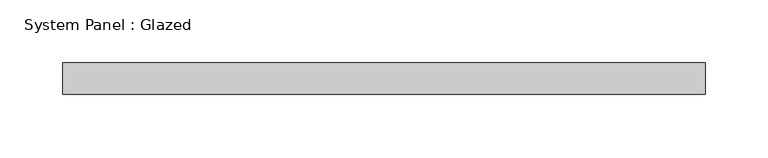
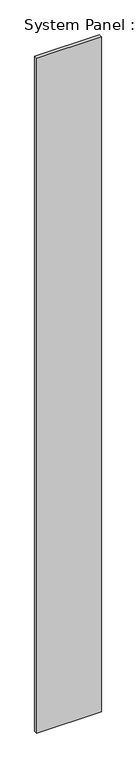
"""IFC4 building model written with IfcOpenShell, lengths in millimetres: plate geometry, System Panel : Glazed."""

from ifc_helpers import new_model, si_unit, origin, origin_with_axes, place, context, project, spatial, polyline, outline, extrude, source, transform, mapped, element, save


def system_panel_glazed_5e2fd105(model_context):
    return source(origin(), model_context, "Body", "SweptSolid", [
        extrude(outline(polyline([(257.175, 19.05), (-257.175, 19.05), (-257.175, 44.45), (257.175, 44.45), (257.175, 19.05)])), origin_with_axes(), (0.0, 0.0, 1.0), 5666.3288504),
    ])


if __name__ == "__main__":
    model = new_model("IFC4")
    model_context = context("Model", 3, world=origin())
    ifc_project = project(units=[si_unit("LENGTHUNIT", "METRE", prefix="MILLI")], contexts=[model_context])
    site = spatial("IfcSite", under=ifc_project)
    building = spatial("IfcBuilding", under=site)
    placement = place(None, origin())
    system_panel_glazed_shape = system_panel_glazed_5e2fd105(model_context)
    element("IfcPlate", 1, ObjectType="System Panel : Glazed", at=placement, inside=building, context=model_context, shape_type="MappedRepresentation", body=[
        mapped(system_panel_glazed_shape, transform((0.0, 0.0, 0.0), x_axis=(1.0, 0.0, 0.0), y_axis=(0.0, 1.0, 0.0), z_axis=(0.0, 0.0, 1.0))),
    ])
    save(model, "model.ifc")

# Revit data of these elements
# Type "System Panel : Glazed"
#   Construction Type Id = "GSP4R"
#   Analytic Construction = "1/8 in Pilkington single glazing"
#   Visual Light Transmittance = 0.9
#   Solar Heat Gain Coefficient = 0.86
#   Heat Transfer Coefficient (U) = 1.18115 BTU/(h·ft²·°F)
#   Define Thermal Properties by = 1
# Element 1 (IfcPlate, "System Panel : Glazed")
#   Materials on its faces: "Glass"
# Materials
#   "Glass": class "Glass", colour RGB 0 128 192, transparency 0.75, Description = "Soda Lime Glass", Cost = 0
